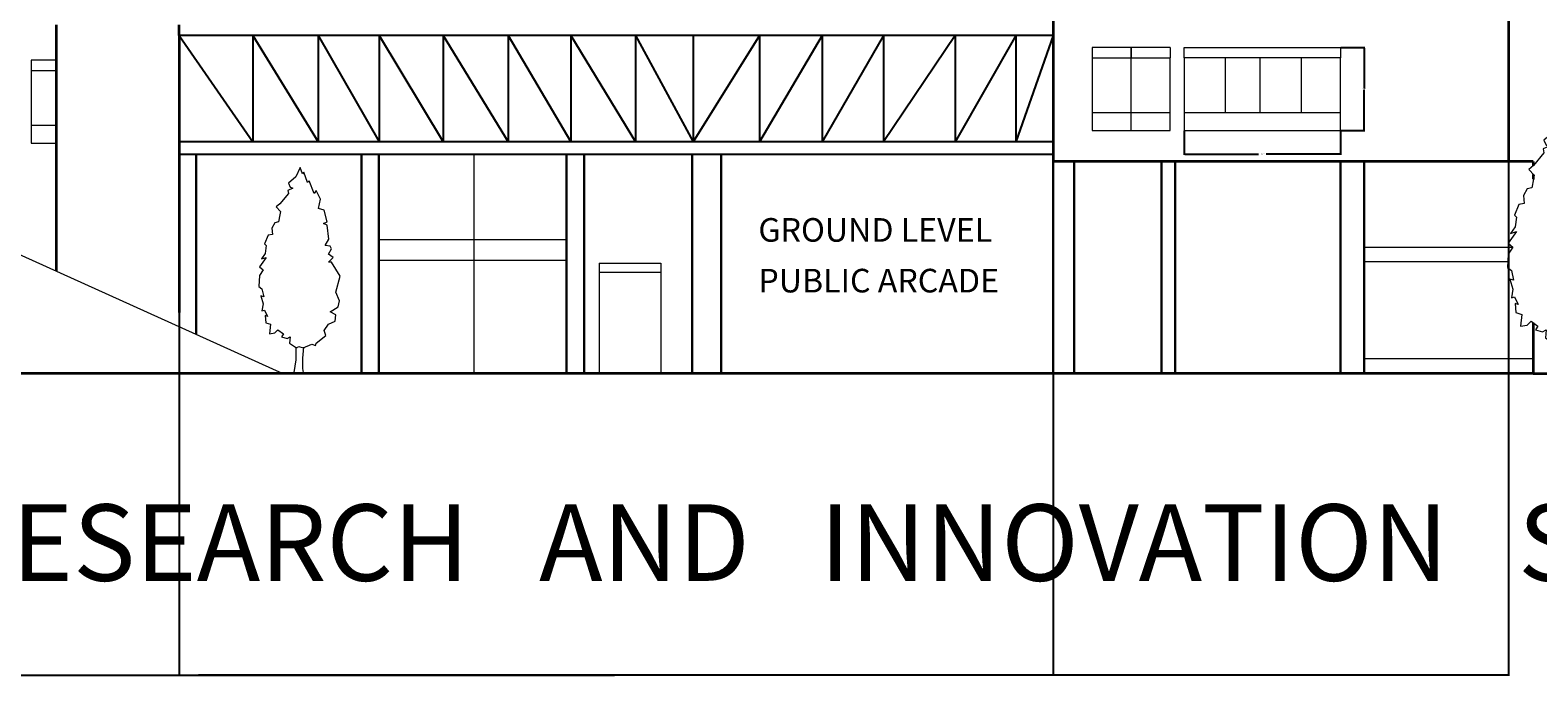
# Model space of a CAD drawing. Units: inches. Extents: x -934 to 898, y -1502 to 444.
# Tile 8 of 10: x -117 to 286, y -260 to -87. Entities that reach past the tile are written whole.
import ezdxf

# ---------------------------------------------------------------- set-up
doc = ezdxf.new("R2010")
doc.units = ezdxf.units.IN
doc.header["$MEASUREMENT"] = 0
for name, color, linetype, lineweight in [('A-ANNO-DIMS', 2, 'Continuous', 18), ('A-ANNO-TEXT', 7, 'Continuous', 18), ('A-ANNO-TITL', 7, 'Continuous', 30), ('A-COLS', 1, 'Continuous', 30), ('A-DOOR', 3, 'Continuous', 18), ('A-ELEV', 7, 'Continuous', 35), ('A-FLOR-STRS', 7, 'Continuous', 18), ('A-GLAZ', 4, 'Continuous', 13), ('L-GRND', 7, 'Continuous', 35), ('L-PLNT-TREE', 3, 'Continuous', 13), ('S-BRDG', 5, 'Continuous', 25)]:
    doc.layers.add(name, color=color, linetype=linetype, lineweight=lineweight)
doc.styles.get("Standard").update_dxf_attribs({"font": 'arial.ttf'})
doc.dimstyles.get("Standard").update_dxf_attribs({"dimtxt": 0.18, "dimasz": 0.18, "dimexe": 0.18, "dimexo": 0.0625, "dimgap": 0.09, "dimtad": 0, "dimtih": 1, "dimtoh": 1, "dimdec": 4, "dimzin": 0, "dimdsep": 46, "dimtxsty": 'Standard', "dimcen": 0.09, "dimadec": 0, "dimazin": 0, "dimtfac": 1, "dimtdec": 4, "dimtofl": 0, "dimtmove": 0, "dimatfit": 3, "dimfxl": 1, "dimtolj": 1, "dimtzin": 0, "dimarcsym": 0})

# ---------------------------------------------------------------- blocks, each defined once
blk = doc.blocks.new('*U5')
blk.add_lwpolyline([(-2.754, 191.699), (-6.78, 182.851), (-13.682, 176.953), (-11.956, 173.266), (-9.656, 172.529), (-14.257, 170.317), (-13.682, 167.368), (-21.733, 157.783), (-25.184, 154.834), (-21.158, 150.41), (-21.733, 147.461), (-22.884, 140.825), (-26.334, 140.087), (-29.21, 134.926), (-28.635, 129.028), (-32.661, 128.291), (-36.111, 120.18), (-34.386, 118.706), (-35.536, 111.333), (-38.987, 106.171), (-34.386, 107.646), (-40.712, 98.798), (-37.261, 95.849), (-40.712, 90.688), (-41.287, 80.366), (-38.412, 78.154), (-36.686, 70.781), (-39.562, 71.518), (-37.261, 64.145), (-38.412, 57.509), (-36.111, 58.247), (-33.236, 52.348), (-35.536, 53.086), (-34.961, 46.45), (-30.36, 44.975), (-31.51, 36.128), (-26.334, 36.865), (-23.459, 39.814), (-18.283, 36.128), (-20.008, 33.178), (-14.832, 31.704), (-11.956, 33.178), (-12.531, 27.28), (-6.205, 22.856), (-3.905, 24.331), (0.121, 22.856), (8.173, 26.543), (11.624, 25.068), (12.199, 27.28), (21.4, 34.653), (19.675, 39.077), (23.701, 44.975), (30.027, 47.924), (30.602, 53.823), (25.426, 56.772), (32.903, 61.196), (34.053, 67.094), (30.602, 75.205), (34.628, 89.951), (26.576, 103.222), (23.701, 103.222), (28.302, 107.646), (23.701, 110.595), (26.576, 115.756), (25.426, 117.968), (20.825, 118.706), (24.276, 124.604), (22.551, 137.876), (19.1, 139.35), (22.551, 140.825), (19.675, 151.884), (14.499, 153.359), (16.224, 162.207), (12.199, 170.317), (10.473, 167.368), (5.872, 179.165), (4.147, 177.69), (0.696, 187.275), (-0.454, 185.8)], close=True)
for points in [[(-6.813, 23.669), (-6.813, 11.669), (-8.627, 0)], [(0.387, 23.669), (-0.576, 13.271), (-0.576, 3.686), (0, 0)]]:
    blk.add_lwpolyline(points)
blk = doc.blocks.new('WIN-TWIN-NARROW')
for p, q in [((10.5, 22.21), (0, 22.21)), ((0, 22.21), (0, 19.45)), ((20.91, 22.21), (10.41, 22.21)), ((10.41, 22.21), (10.41, 19.45)), ((10.5, 22.21), (10.5, 19.45)), ((20.91, 22.21), (20.91, 19.45)), ((0, 19.45), (0, 4.84)), ((0, 19.45), (10.5, 19.45)), ((10.41, 19.45), (10.41, 4.84)), ((10.41, 19.45), (20.91, 19.45)), ((10.5, 4.84), (10.5, 19.45)), ((20.91, 4.84), (20.91, 19.45)), ((0, 4.84), (10.5, 4.84)), ((0, 4.84), (0, 0)), ((10.41, 4.84), (20.91, 4.84)), ((10.41, 4.84), (10.41, 0)), ((10.5, 0), (10.5, 4.84)), ((20.91, 0), (20.91, 4.84)), ((0, 0), (10.5, 0)), ((10.41, 0), (20.91, 0))]:
    blk.add_line(p, q)
blk = doc.blocks.new('WIN-RIBBON-LARGE')
for p, q in [((0, 19.45), (0, 22.21)), ((0, 22.21), (41.85, 22.21)), ((41.85, 22.21), (41.85, 19.45)), ((0, 19.45), (0, 4.84)), ((41.85, 19.45), (0, 19.45)), ((10.96, 19.45), (10.96, 4.84)), ((20.23, 19.45), (20.23, 4.84)), ((31.34, 19.45), (31.34, 4.84)), ((41.85, 4.84), (41.85, 19.45)), ((0, 4.84), (41.85, 4.84)), ((0, 4.84), (0, 0)), ((41.85, 0), (41.85, 4.84)), ((0, 0), (41.85, 0))]:
    blk.add_line(p, q)
blk = doc.blocks.new('*D39')
at = {"layer": 'A-ANNO-DIMS', "color": 0, "lineweight": -2, "transparency": 16777216}
for p, q in [((191.47, -113.77), (191.47, -120.16)), ((233.32, -113.77), (233.32, -120.16)), ((191.65, -119.98), (211.36, -119.98)), ((233.14, -119.98), (213.44, -119.98))]:
    blk.add_line(p, q, dxfattribs=at)
at = {"layer": 'A-ANNO-DIMS', "color": 0, "transparency": 16777216}
for points in [[(191.65, -119.95), (191.65, -120.01), (191.47, -119.98)], [(233.14, -119.95), (233.14, -120.01), (233.32, -119.98)]]:
    blk.add_solid(points, dxfattribs=at)
at = {"layer": 'Defpoints', "color": 0, "transparency": 16777216}
for p in [(191.47, -113.71), (233.32, -113.71), (233.32, -119.98)]:
    blk.add_point(p, dxfattribs=at)
at = {"layer": 'A-ANNO-DIMS', "color": 0, "transparency": 16777216, "insert": (212.4, -119.98), "char_height": 0.18, "attachment_point": 5}
blk.add_mtext('\\A1;RIBBON 42 TYP.', dxfattribs=at)
blk = doc.blocks.new('*D40')
at = {"layer": 'A-ANNO-DIMS', "color": 0, "lineweight": -2, "transparency": 16777216}
for p, q in [((233.38, -91.5), (239.78, -91.5)), ((239.6, -91.68), (239.6, -102.42)), ((239.6, -113.53), (239.6, -102.78)), ((233.38, -113.71), (239.78, -113.71))]:
    blk.add_line(p, q, dxfattribs=at)
at = {"layer": 'A-ANNO-DIMS', "color": 0, "transparency": 16777216}
for points in [[(239.57, -91.68), (239.63, -91.68), (239.6, -91.5)], [(239.57, -113.53), (239.63, -113.53), (239.6, -113.71)]]:
    blk.add_solid(points, dxfattribs=at)
at = {"layer": 'Defpoints', "color": 0, "transparency": 16777216}
for p in [(233.32, -91.5), (239.6, -91.5), (233.32, -113.71)]:
    blk.add_point(p, dxfattribs=at)
at = {"layer": 'A-ANNO-DIMS', "color": 0, "transparency": 16777216, "insert": (239.6, -102.6), "char_height": 0.18, "attachment_point": 5}
blk.add_mtext('\\A1;22 TYP.', dxfattribs=at)
blk = doc.blocks.new('*D79')
at = {"layer": 'A-ANNO-DIMS', "color": 0, "lineweight": -2, "transparency": 16777216}
for p, q in [((278.23, -122.09), (278.23, -259.51)), ((-423.28, -178.74), (-423.28, -259.51)), ((-423.1, -259.33), (-72.92, -259.33)), ((278.05, -259.33), (-72.13, -259.33))]:
    blk.add_line(p, q, dxfattribs=at)
at = {"layer": 'A-ANNO-DIMS', "color": 0, "transparency": 16777216}
for points in [[(-423.1, -259.3), (-423.1, -259.36), (-423.28, -259.33)], [(278.05, -259.3), (278.05, -259.36), (278.23, -259.33)]]:
    blk.add_solid(points, dxfattribs=at)
at = {"layer": 'Defpoints', "color": 0, "transparency": 16777216}
for p in [(278.23, -122.02), (-423.28, -178.68), (278.23, -259.33)]:
    blk.add_point(p, dxfattribs=at)
at = {"layer": 'A-ANNO-DIMS', "color": 0, "transparency": 16777216, "insert": (-72.53, -259.33), "char_height": 0.18, "attachment_point": 5}
blk.add_mtext('\\A1;701.5', dxfattribs=at)
blk = doc.blocks.new('*D80')
at = {"layer": 'A-ANNO-DIMS', "color": 0, "lineweight": -2, "transparency": 16777216}
for p, q in [((261.62, 129.1), (464.31, 129.1)), ((464.13, 128.92), (464.13, -24.61)), ((464.13, -178.5), (464.13, -24.97)), ((239.7, -178.68), (464.31, -178.68))]:
    blk.add_line(p, q, dxfattribs=at)
at = {"layer": 'A-ANNO-DIMS', "color": 0, "transparency": 16777216}
for points in [[(464.1, 128.92), (464.16, 128.92), (464.13, 129.1)], [(464.1, -178.5), (464.16, -178.5), (464.13, -178.68)]]:
    blk.add_solid(points, dxfattribs=at)
at = {"layer": 'Defpoints', "color": 0, "transparency": 16777216}
for p in [(261.56, 129.1), (464.13, 129.1), (239.64, -178.68)]:
    blk.add_point(p, dxfattribs=at)
at = {"layer": 'A-ANNO-DIMS', "color": 0, "transparency": 16777216, "insert": (464.13, -24.79), "char_height": 0.18, "attachment_point": 5}
blk.add_mtext('\\A1;307.8', dxfattribs=at)
blk = doc.blocks.new('*D82')
at = {"layer": 'A-ANNO-DIMS', "color": 0, "lineweight": -2, "transparency": 16777216}
for p, q in [((-77.35, -120.21), (-77.35, -259.51)), ((156.42, -120.21), (156.42, -259.51)), ((-77.17, -259.33), (39.14, -259.33)), ((156.24, -259.33), (39.93, -259.33))]:
    blk.add_line(p, q, dxfattribs=at)
at = {"layer": 'A-ANNO-DIMS', "color": 0, "transparency": 16777216}
for points in [[(-77.17, -259.3), (-77.17, -259.36), (-77.35, -259.33)], [(156.24, -259.3), (156.24, -259.36), (156.42, -259.33)]]:
    blk.add_solid(points, dxfattribs=at)
at = {"layer": 'Defpoints', "color": 0, "transparency": 16777216}
for p in [(-77.35, -120.14), (156.42, -120.14), (156.42, -259.33)]:
    blk.add_point(p, dxfattribs=at)
at = {"layer": 'A-ANNO-DIMS', "color": 0, "transparency": 16777216, "insert": (39.53, -259.33), "char_height": 0.18, "attachment_point": 5}
blk.add_mtext('\\A1;233.8', dxfattribs=at)

msp = doc.modelspace()

# ---------------------------------------------------------------- linework, layer by layer
at = {"layer": 'A-COLS'}
for p, q in [((-72.829, -120.144), (-72.829, -168.1991)), ((-28.6063, -120.144), (-28.6063, -178.6804)), ((-23.9442, -120.144), (-23.9442, -178.6804)), ((26.3021, -120.144), (26.3021, -178.6804)), ((30.9641, -120.144), (30.9641, -178.6804)), ((59.8691, -120.144), (59.8691, -178.6804)), ((67.6239, -120.144), (67.6239, -178.6804)), ((156.4222, -122.024), (156.4222, -178.6804)), ((162.0991, -122.024), (162.0991, -178.6804)), ((185.4254, -122.024), (185.4254, -178.6804)), ((189.0424, -122.024), (189.0424, -178.6804)), ((233.3209, -122.024), (233.3209, -178.6804)), ((239.6401, -178.6804), (239.6401, -122.024))]:
    msp.add_line(p, q, dxfattribs=at)
at = {"layer": 'A-DOOR'}
for p, q in [((35.0463, -149.1597), (51.4984, -149.1597)), ((35.0463, -149.1597), (35.0463, -178.6804)), ((51.4984, -149.1597), (51.4984, -178.6804)), ((35.0463, -151.5974), (51.4984, -151.5974))]:
    msp.add_line(p, q, dxfattribs=at)
at = {"layer": 'A-ELEV'}
for p, q in [((156.4222, -82.9144), (156.4222, -122.024)), ((278.229, -82.924), (278.229, -122.024)), ((-110.2409, -85.4234), (-110.2409, -151.3215)), ((-77.3547, -88.3005), (-77.3547, -85.4234)), ((-77.3547, -88.3005), (-77.3547, -162.3396)), ((278.229, -122.024), (156.4222, -122.024)), ((284.8904, -122.024), (274.6175, -122.024)), ((278.229, -122.024), (278.229, -122.024)), ((278.229, -122.024), (278.229, -122.024)), ((278.229, -122.024), (278.229, -122.024)), ((284.8904, -122.024), (284.8904, -123.0507)), ((284.8904, -125.415), (284.8904, -126.7283)), ((284.8904, -165.0972), (284.8904, -178.6804))]:
    msp.add_line(p, q, dxfattribs=at)
at = {"layer": 'A-FLOR-STRS'}
for p, q in [((-202.6582, -109.6295), (-49.5955, -178.6804)), ((-77.3547, -162.3396), (-77.3547, -166.1574))]:
    msp.add_line(p, q, dxfattribs=at)
at = {"layer": 'A-GLAZ'}
for p, q in [((-110.2409, -94.87), (-116.8962, -94.87)), ((-116.8962, -94.87), (-116.8962, -97.6249)), ((-116.8962, -97.6249), (-116.8962, -112.2432)), ((-116.8962, -97.6249), (-110.2409, -97.6249)), ((-116.8962, -112.2432), (-110.2409, -112.2432)), ((-116.8962, -112.2432), (-116.8962, -117.0786)), ((-116.8962, -117.0786), (-110.2409, -117.0786)), ((1.4651, -120.144), (1.4651, -178.6804)), ((-23.9442, -142.8388), (26.3021, -142.8388)), ((239.6401, -144.9035), (279.4146, -144.9035)), ((-23.9442, -148.3901), (26.3021, -148.3901)), ((239.6401, -148.7032), (278.0906, -148.7032)), ((239.6401, -174.6887), (284.8904, -174.6887))]:
    msp.add_line(p, q, dxfattribs=at)
at = {"layer": 'L-GRND'}
for q in [(-573.1189, -178.6804), (408.8772, -178.6804)]:
    msp.add_line((284.8904, -178.6804), q, dxfattribs=at)
at = {"layer": 'S-BRDG'}
for p, q in [((-25.055, -88.3005), (-77.3547, -88.3005)), ((-77.3547, -88.3005), (-57.6755, -116.749)), ((-57.6755, -88.3005), (-57.6755, -116.749)), ((-57.6755, -88.3005), (-40.1321, -116.749)), ((-40.1321, -88.3005), (-40.1321, -116.749)), ((-40.1321, -88.3005), (-23.8583, -116.749)), ((71.4232, -88.3005), (-25.055, -88.3005)), ((-23.8583, -88.3005), (-23.8583, -116.749)), ((-23.8583, -88.3005), (-6.7427, -116.749)), ((-6.7427, -88.3005), (-6.7427, -116.749)), ((-6.7427, -88.3005), (10.6852, -116.749)), ((10.6852, -88.3005), (10.6852, -116.749)), ((10.6852, -88.3005), (27.4207, -116.749)), ((27.4207, -88.3005), (27.4207, -116.749)), ((27.4207, -88.3005), (44.7672, -116.749)), ((44.7672, -88.3005), (44.7672, -116.749)), ((44.7672, -88.3005), (60.1176, -116.749)), ((60.1176, -88.3005), (60.1176, -116.749)), ((77.9228, -88.3005), (60.1176, -116.749)), ((156.4222, -88.3005), (71.4232, -88.3005)), ((77.9228, -88.3005), (77.9228, -116.749)), ((94.6582, -88.3005), (77.9228, -116.749)), ((94.6582, -88.3005), (94.6582, -116.749)), ((111.0474, -88.3005), (94.6582, -116.749)), ((111.0474, -88.3005), (111.0474, -116.749)), ((130.2066, -88.3005), (111.0474, -116.749)), ((130.2066, -88.3005), (130.2066, -116.749)), ((146.4804, -88.3005), (130.2066, -116.749)), ((146.4804, -88.3005), (146.4804, -116.749)), ((156.4222, -88.3005), (146.4804, -116.749)), ((74.4978, -116.749), (-77.3547, -116.749)), ((156.4222, -116.749), (74.4978, -116.749)), ((85.5397, -120.144), (-77.3547, -120.144)), ((156.4222, -120.144), (85.5397, -120.144))]:
    msp.add_line(p, q, dxfattribs=at)

# ---------------------------------------------------------------- block references
at = {"layer": 'A-GLAZ'}
for name, p in [('WIN-TWIN-NARROW', (166.852, -113.7231)), ('WIN-RIBBON-LARGE', (191.4748, -113.7072))]:
    msp.add_blockref(name, p, dxfattribs=at)
at = {"layer": 'L-PLNT-TREE'}
for p, xscale, yscale, zscale in [((292.566, -178.7166), 0.3528399638811642, 0.3528399638811642, 0.3528399638811642), ((-44.2121, -178.3705), 0.2857357741909547, 0.2857357741909547, 0.2857357741909547)]:
    msp.add_blockref('*U5', p, dxfattribs=dict(at, xscale=xscale, yscale=yscale, zscale=zscale))

# ---------------------------------------------------------------- texts
at = {"layer": 'A-ANNO-TEXT'}
for s, p in [('GROUND LEVEL', (77.5937, -143.4287)), ('PUBLIC ARCADE', (77.5937, -156.9932))]:
    msp.add_text(s, height=6.31231, dxfattribs=at).set_placement(p)
at = {"layer": 'A-ANNO-TITL'}
msp.add_text('LINEAR   CAMPUS   AXIS ELEVATION   RESEARCH   AND   INNOVATION   SPINE ', height=20.457511, dxfattribs=at).set_placement((-613.4854, -234.1138))

# ---------------------------------------------------------------- dimensions: what is measured, and where the dimension line sits
at = {"layer": 'A-ANNO-DIMS'}
dim = msp.add_linear_dim(base=(464.1272, 129.1024), p1=(239.6401, -178.6804), p2=(261.5611, 129.1024), angle=90, dimstyle='Standard', override={"dimdec": 1, "dimlfac": 1, "dimrnd": 0, "dimzin": 0, "dimdsep": 46, "dimlunit": 2}, dxfattribs=at)
dim.commit()
dim.dimension.update_dxf_attribs({"geometry": '*D80', "text_midpoint": (464.1272, -24.789)})
dim = msp.add_linear_dim(base=(239.5978, -91.4986), p1=(233.3209, -113.7072), p2=(233.3209, -91.4986), angle=90, text='<> TYP.', dimstyle='Standard', override={"dimdec": 0, "dimlfac": 1, "dimrnd": 0, "dimzin": 0, "dimdsep": 46, "dimlunit": 2}, dxfattribs=at)
dim.commit()
dim.dimension.update_dxf_attribs({"geometry": '*D40', "text_midpoint": (239.5978, -102.6029)})
dim = msp.add_linear_dim(base=(233.3209, -119.9841), p1=(191.4748, -113.7072), p2=(233.3209, -113.7072), text='RIBBON <> TYP.', dimstyle='Standard', override={"dimdec": 0, "dimlfac": 1, "dimrnd": 0, "dimzin": 0, "dimdsep": 46, "dimlunit": 2}, dxfattribs=at)
dim.commit()
dim.dimension.update_dxf_attribs({"geometry": '*D39', "text_midpoint": (212.3979, -119.9841)})
for base, p1, p2, picture, middle in [((156.4222, -259.3312), (-77.3547, -120.144), (156.4222, -120.144), '*D82', (39.5338, -259.3312)), ((278.229, -259.3312), (-423.2792, -178.6804), (278.229, -122.024), '*D79', (-72.5251, -259.3312))]:
    dim = msp.add_linear_dim(base=base, p1=p1, p2=p2, dimstyle='Standard', override={"dimdec": 1, "dimlfac": 1, "dimrnd": 0, "dimzin": 0, "dimdsep": 46, "dimlunit": 2}, dxfattribs=at)
    dim.commit()
    dim.dimension.update_dxf_attribs({"geometry": picture, "text_midpoint": middle})

doc.saveas('drawing.dxf')
